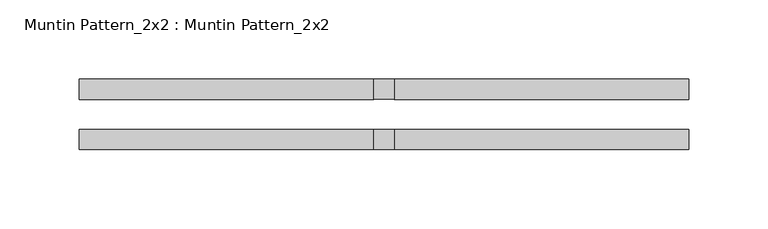
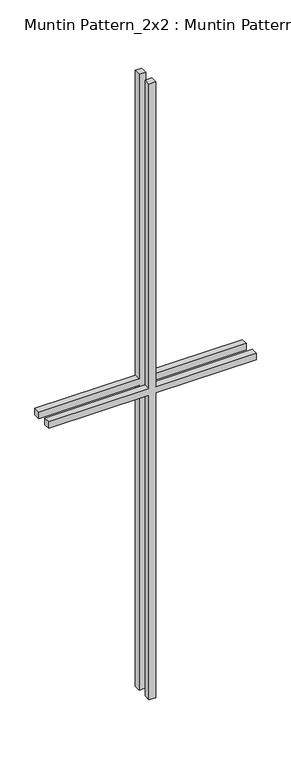
"""IFC4 building model written with IfcOpenShell, lengths in millimetres: proxy geometry, Muntin Pattern_2x2 : Muntin Pattern_2x2."""

from ifc_helpers import new_model, si_unit, frame, origin, place, context, project, spatial, polyline, outline, extrude, source, transform, mapped, element, save


def muntin_pattern_2x2_muntin_pattern_2x2_88bf7f41(model_context):
    return source(origin(), model_context, "Body", "SweptSolid", [
        extrude(outline(polyline([(609.6, -6.35), (609.6, -192.0875), (596.9, -192.0875), (596.9, -6.35), (0.0, -6.35), (0.0, 6.35), (596.9, 6.35), (596.9, 192.0875), (609.6, 192.0875), (609.6, 6.35), (1206.5, 6.35), (1206.5, -6.35), (609.6, -6.35)])), frame((0.0, 9.525, 0.0), z_axis=(0.0, 1.0, 0.0), x_axis=(0.0, 0.0, 1.0)), (0.0, 0.0, 1.0), 12.7),
        extrude(outline(polyline([(609.6, -6.35), (609.6, -192.0875), (596.9, -192.0875), (596.9, -6.35), (0.0, -6.35), (0.0, 6.35), (596.9, 6.35), (596.9, 192.0875), (609.6, 192.0875), (609.6, 6.35), (1206.5, 6.35), (1206.5, -6.35), (609.6, -6.35)])), frame((0.0, -22.225, 0.0), z_axis=(0.0, 1.0, 0.0), x_axis=(0.0, 0.0, 1.0)), (0.0, 0.0, 1.0), 12.7),
    ])


if __name__ == "__main__":
    model = new_model("IFC4")
    model_context = context("Model", 3, world=origin())
    ifc_project = project(units=[si_unit("LENGTHUNIT", "METRE", prefix="MILLI")], contexts=[model_context])
    site = spatial("IfcSite", under=ifc_project)
    building = spatial("IfcBuilding", under=site)
    placement = place(None, origin())
    muntin_pattern_2x2_muntin_pattern_2x2_shape = muntin_pattern_2x2_muntin_pattern_2x2_88bf7f41(model_context)
    element("IfcBuildingElementProxy", 1, Name="Muntin Pattern_2x2 : Muntin Pattern_2x2", ObjectType="Muntin Pattern_2x2 : Muntin Pattern_2x2", at=placement, inside=building, context=model_context, shape_type="MappedRepresentation", body=[
        mapped(muntin_pattern_2x2_muntin_pattern_2x2_shape, transform((0.0, 0.0, 0.0), x_axis=(1.0, 0.0, 0.0), y_axis=(0.0, 1.0, 0.0), z_axis=(0.0, 0.0, 1.0))),
    ])
    save(model, "model.ifc")

# Revit data of these elements
# Type "Muntin Pattern_2x2 : Muntin Pattern_2x2"
#   Width [instance default] = 4' - 0"
#   Thickness = 0' - 0 1/2"
#   Height [instance default] = 4' - 0"
#   Distance = 0' - 0 3/4"
#   Interior Material [instance default] = none
#   Exterior Material [instance default] = none
#   Default Elevation = 0
# Element 1 (IfcBuildingElementProxy, "Muntin Pattern_2x2 : Muntin Pattern_2x2")
#   Width = 1' - 3 1/8"
#   Height = 3' - 11 1/2"
#   Interior Material = Wood - Stained
#   Exterior Material = Clad - White
#   Materials on its faces: "Clad - White", "Wood - Stained"
# Materials
#   "Clad - White": class "Wood", colour RGB 30 30 30, transparency 0, Cost = 0
#   "Wood - Stained": class "Wood", colour RGB 224 178 126, transparency 0, Cost = 0
